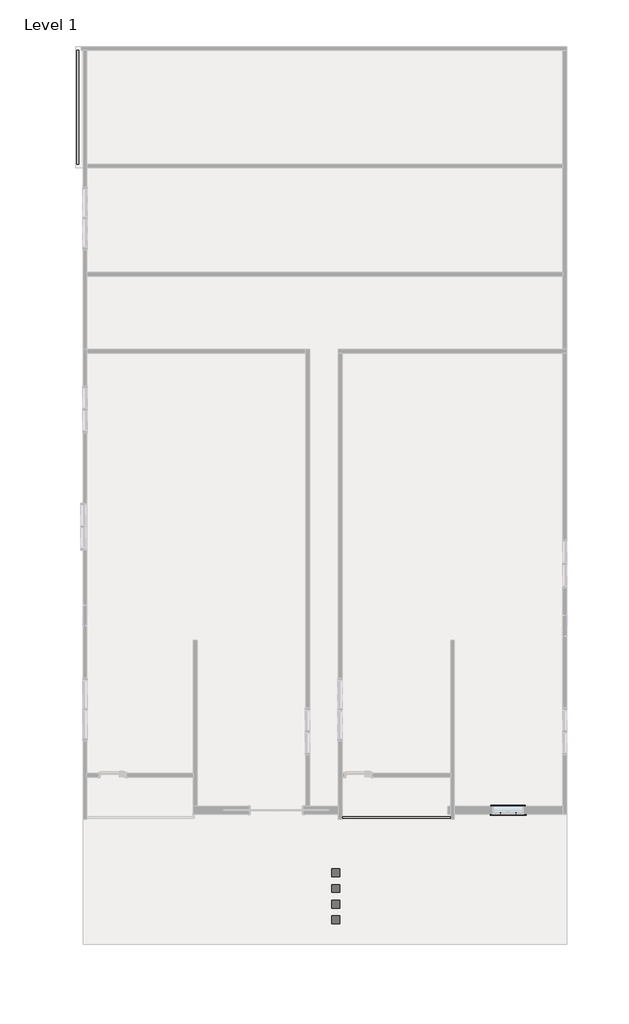
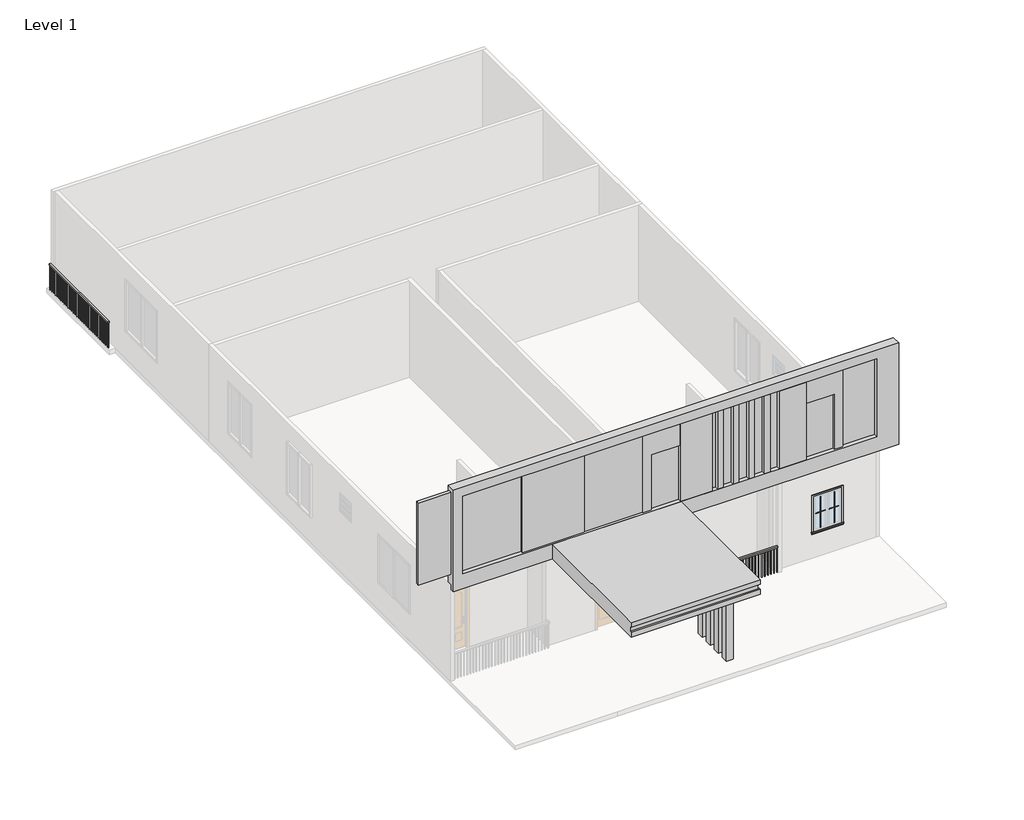
# One storey, part 3 of 3: 5 proxies, 3 railings.
"""IFC4 building model written with IfcOpenShell, lengths in millimetres."""

from ifc_helpers import new_model, si_unit, frame, origin, origin_with_axes, place, context, project, spatial, polyline, outline, extrude, transform, mapped, element, save
from components import generic_models_1_generic_models_1_486b888d, muntin_pattern_2x2_muntin_pattern_2x2_1acec82f, muntin_pattern_2x2_muntin_pattern_2x2_43d02eee, trim_window_exterior_flat_with_sill_e4b28ec3, trim_window_interior_flat_picture_frame_39ff4276

model = new_model("IFC4")

# Units and contexts
model_context = context("Model", 3, world=origin())
ifc_project = project(units=[si_unit("LENGTHUNIT", "METRE", prefix="MILLI")], contexts=[model_context])

# Site, building, storey
site = spatial("IfcSite", under=ifc_project)
building = spatial("IfcBuilding", under=site)
storey = spatial("IfcBuildingStorey", under=building, Name="Level 1", Elevation=0.0)

# Proxies
placement = place(None, origin())
generic_models_1_generic_models_1_shape = generic_models_1_generic_models_1_486b888d(model_context)
element("IfcBuildingElementProxy", 1, Name="Generic Models 1 : Generic Models 1", ObjectType="Generic Models 1 : Generic Models 1", at=placement, inside=storey, context=model_context, shape_type="MappedRepresentation", body=[
    mapped(generic_models_1_generic_models_1_shape, transform((0.0, 0.0, 0.0), x_axis=(1.0, 0.0, 0.0), y_axis=(0.0, 1.0, 0.0), z_axis=(0.0, 0.0, 1.0))),
])
muntin_pattern_2x2_muntin_pattern_2x2_shape = muntin_pattern_2x2_muntin_pattern_2x2_1acec82f(model_context)
element("IfcBuildingElementProxy", 2, Name="Muntin Pattern_2x2 : Muntin Pattern_2x2", ObjectType="Muntin Pattern_2x2 : Muntin Pattern_2x2", at=placement, inside=storey, context=model_context, shape_type="MappedRepresentation", body=[
    mapped(muntin_pattern_2x2_muntin_pattern_2x2_shape, transform((4424.1833786, -10576.3529557, 984.25), x_axis=(-1.0, 0.0, 0.0), y_axis=(0.0, -1.0, 0.0), z_axis=(0.0, 0.0, 1.0))),
])
muntin_pattern_2x2_muntin_pattern_2x2_2_shape = muntin_pattern_2x2_muntin_pattern_2x2_43d02eee(model_context)
element("IfcBuildingElementProxy", 3, Name="Muntin Pattern_2x2 : Muntin Pattern_2x2", ObjectType="Muntin Pattern_2x2 : Muntin Pattern_2x2", at=placement, inside=storey, context=model_context, shape_type="MappedRepresentation", body=[
    mapped(muntin_pattern_2x2_muntin_pattern_2x2_2_shape, transform((3970.1583786, -10576.3529557, 984.25), x_axis=(1.0, 0.0, 0.0), y_axis=(0.0, 1.0, 0.0), z_axis=(0.0, 0.0, 1.0))),
])
trim_window_exterior_flat_with_sill_shape = trim_window_exterior_flat_with_sill_e4b28ec3(model_context)
element("IfcBuildingElementProxy", 4, Name="Trim-Window-Exterior-Flat : with Sill", ObjectType="Trim-Window-Exterior-Flat : with Sill", at=placement, inside=storey, context=model_context, shape_type="MappedRepresentation", body=[
    mapped(trim_window_exterior_flat_with_sill_shape, transform((4197.1708786, -10585.8779557, 2133.6), x_axis=(1.0, 0.0, 0.0), y_axis=(0.0, 0.0, 1.0), z_axis=(0.0, -1.0, 0.0))),
])
trim_window_interior_flat_picture_frame_shape = trim_window_interior_flat_picture_frame_39ff4276(model_context)
element("IfcBuildingElementProxy", 5, Name="Trim-Window-Interior-Flat : Picture Frame", ObjectType="Trim-Window-Interior-Flat : Picture Frame", at=placement, inside=storey, context=model_context, shape_type="MappedRepresentation", body=[
    mapped(trim_window_interior_flat_picture_frame_shape, transform((4197.1708786, -10357.2779557, 2133.6), x_axis=(-1.0, 0.0, 0.0), y_axis=(0.0, 0.0, 1.0), z_axis=(0.0, 1.0, 0.0))),
])

# Railings
element("IfcRailing", 6, ObjectType="Handrail - Rectangular", at=placement, inside=storey, context=model_context, shape_type="SweptSolid", body=[
    extrude(outline(polyline([(-648.5431282, -10709.8005933), (-648.5431282, -10659.0005933), (2515.990751, -10659.0005933), (2515.990751, -10709.8005933), (-648.5431282, -10709.8005933)])), frame((0.0, 0.0, 863.6), z_axis=(0.0, 0.0, 1.0), x_axis=(1.0, 0.0, 0.0)), (0.0, 0.0, 1.0), 50.8),
    extrude(outline(polyline([(2491.5318718, -10693.9255933), (2491.5318718, -10674.8755933), (2510.5818718, -10674.8755933), (2510.5818718, -10693.9255933), (2491.5318718, -10693.9255933)])), origin_with_axes(), (0.0, 0.0, 1.0), 863.6),
    extrude(outline(polyline([(2389.9318718, -10693.9255933), (2389.9318718, -10674.8755933), (2408.9818718, -10674.8755933), (2408.9818718, -10693.9255933), (2389.9318718, -10693.9255933)])), origin_with_axes(), (0.0, 0.0, 1.0), 863.6),
    extrude(outline(polyline([(2288.3318718, -10693.9255933), (2288.3318718, -10674.8755933), (2307.3818718, -10674.8755933), (2307.3818718, -10693.9255933), (2288.3318718, -10693.9255933)])), origin_with_axes(), (0.0, 0.0, 1.0), 863.6),
    extrude(outline(polyline([(2186.7318718, -10693.9255933), (2186.7318718, -10674.8755933), (2205.7818718, -10674.8755933), (2205.7818718, -10693.9255933), (2186.7318718, -10693.9255933)])), origin_with_axes(), (0.0, 0.0, 1.0), 863.6),
    extrude(outline(polyline([(2085.1318718, -10693.9255933), (2085.1318718, -10674.8755933), (2104.1818718, -10674.8755933), (2104.1818718, -10693.9255933), (2085.1318718, -10693.9255933)])), origin_with_axes(), (0.0, 0.0, 1.0), 863.6),
    extrude(outline(polyline([(1983.5318718, -10693.9255933), (1983.5318718, -10674.8755933), (2002.5818718, -10674.8755933), (2002.5818718, -10693.9255933), (1983.5318718, -10693.9255933)])), origin_with_axes(), (0.0, 0.0, 1.0), 863.6),
    extrude(outline(polyline([(1881.9318718, -10693.9255933), (1881.9318718, -10674.8755933), (1900.9818718, -10674.8755933), (1900.9818718, -10693.9255933), (1881.9318718, -10693.9255933)])), origin_with_axes(), (0.0, 0.0, 1.0), 863.6),
    extrude(outline(polyline([(1780.3318718, -10693.9255933), (1780.3318718, -10674.8755933), (1799.3818718, -10674.8755933), (1799.3818718, -10693.9255933), (1780.3318718, -10693.9255933)])), origin_with_axes(), (0.0, 0.0, 1.0), 863.6),
    extrude(outline(polyline([(1678.7318718, -10693.9255933), (1678.7318718, -10674.8755933), (1697.7818718, -10674.8755933), (1697.7818718, -10693.9255933), (1678.7318718, -10693.9255933)])), origin_with_axes(), (0.0, 0.0, 1.0), 863.6),
    extrude(outline(polyline([(1577.1318718, -10693.9255933), (1577.1318718, -10674.8755933), (1596.1818718, -10674.8755933), (1596.1818718, -10693.9255933), (1577.1318718, -10693.9255933)])), origin_with_axes(), (0.0, 0.0, 1.0), 863.6),
    extrude(outline(polyline([(1475.5318718, -10693.9255933), (1475.5318718, -10674.8755933), (1494.5818718, -10674.8755933), (1494.5818718, -10693.9255933), (1475.5318718, -10693.9255933)])), origin_with_axes(), (0.0, 0.0, 1.0), 863.6),
    extrude(outline(polyline([(1373.9318718, -10693.9255933), (1373.9318718, -10674.8755933), (1392.9818718, -10674.8755933), (1392.9818718, -10693.9255933), (1373.9318718, -10693.9255933)])), origin_with_axes(), (0.0, 0.0, 1.0), 863.6),
    extrude(outline(polyline([(1272.3318718, -10693.9255933), (1272.3318718, -10674.8755933), (1291.3818718, -10674.8755933), (1291.3818718, -10693.9255933), (1272.3318718, -10693.9255933)])), origin_with_axes(), (0.0, 0.0, 1.0), 863.6),
    extrude(outline(polyline([(1170.7318718, -10693.9255933), (1170.7318718, -10674.8755933), (1189.7818718, -10674.8755933), (1189.7818718, -10693.9255933), (1170.7318718, -10693.9255933)])), origin_with_axes(), (0.0, 0.0, 1.0), 863.6),
    extrude(outline(polyline([(1069.1318718, -10693.9255933), (1069.1318718, -10674.8755933), (1088.1818718, -10674.8755933), (1088.1818718, -10693.9255933), (1069.1318718, -10693.9255933)])), origin_with_axes(), (0.0, 0.0, 1.0), 863.6),
    extrude(outline(polyline([(967.5318718, -10693.9255933), (967.5318718, -10674.8755933), (986.5818718, -10674.8755933), (986.5818718, -10693.9255933), (967.5318718, -10693.9255933)])), origin_with_axes(), (0.0, 0.0, 1.0), 863.6),
    extrude(outline(polyline([(865.9318718, -10693.9255933), (865.9318718, -10674.8755933), (884.9818718, -10674.8755933), (884.9818718, -10693.9255933), (865.9318718, -10693.9255933)])), origin_with_axes(), (0.0, 0.0, 1.0), 863.6),
    extrude(outline(polyline([(764.3318718, -10693.9255933), (764.3318718, -10674.8755933), (783.3818718, -10674.8755933), (783.3818718, -10693.9255933), (764.3318718, -10693.9255933)])), origin_with_axes(), (0.0, 0.0, 1.0), 863.6),
    extrude(outline(polyline([(662.7318718, -10693.9255933), (662.7318718, -10674.8755933), (681.7818718, -10674.8755933), (681.7818718, -10693.9255933), (662.7318718, -10693.9255933)])), origin_with_axes(), (0.0, 0.0, 1.0), 863.6),
    extrude(outline(polyline([(561.1318718, -10693.9255933), (561.1318718, -10674.8755933), (580.1818718, -10674.8755933), (580.1818718, -10693.9255933), (561.1318718, -10693.9255933)])), origin_with_axes(), (0.0, 0.0, 1.0), 863.6),
    extrude(outline(polyline([(459.5318718, -10693.9255933), (459.5318718, -10674.8755933), (478.5818718, -10674.8755933), (478.5818718, -10693.9255933), (459.5318718, -10693.9255933)])), origin_with_axes(), (0.0, 0.0, 1.0), 863.6),
    extrude(outline(polyline([(357.9318718, -10693.9255933), (357.9318718, -10674.8755933), (376.9818718, -10674.8755933), (376.9818718, -10693.9255933), (357.9318718, -10693.9255933)])), origin_with_axes(), (0.0, 0.0, 1.0), 863.6),
    extrude(outline(polyline([(256.3318718, -10693.9255933), (256.3318718, -10674.8755933), (275.3818718, -10674.8755933), (275.3818718, -10693.9255933), (256.3318718, -10693.9255933)])), origin_with_axes(), (0.0, 0.0, 1.0), 863.6),
    extrude(outline(polyline([(154.7318718, -10693.9255933), (154.7318718, -10674.8755933), (173.7818718, -10674.8755933), (173.7818718, -10693.9255933), (154.7318718, -10693.9255933)])), origin_with_axes(), (0.0, 0.0, 1.0), 863.6),
    extrude(outline(polyline([(53.1318718, -10693.9255933), (53.1318718, -10674.8755933), (72.1818718, -10674.8755933), (72.1818718, -10693.9255933), (53.1318718, -10693.9255933)])), origin_with_axes(), (0.0, 0.0, 1.0), 863.6),
    extrude(outline(polyline([(-48.4681282, -10693.9255933), (-48.4681282, -10674.8755933), (-29.4181282, -10674.8755933), (-29.4181282, -10693.9255933), (-48.4681282, -10693.9255933)])), origin_with_axes(), (0.0, 0.0, 1.0), 863.6),
    extrude(outline(polyline([(-150.0681282, -10693.9255933), (-150.0681282, -10674.8755933), (-131.0181282, -10674.8755933), (-131.0181282, -10693.9255933), (-150.0681282, -10693.9255933)])), origin_with_axes(), (0.0, 0.0, 1.0), 863.6),
    extrude(outline(polyline([(-251.6681282, -10693.9255933), (-251.6681282, -10674.8755933), (-232.6181282, -10674.8755933), (-232.6181282, -10693.9255933), (-251.6681282, -10693.9255933)])), origin_with_axes(), (0.0, 0.0, 1.0), 863.6),
    extrude(outline(polyline([(-353.2681282, -10693.9255933), (-353.2681282, -10674.8755933), (-334.2181282, -10674.8755933), (-334.2181282, -10693.9255933), (-353.2681282, -10693.9255933)])), origin_with_axes(), (0.0, 0.0, 1.0), 863.6),
    extrude(outline(polyline([(-454.8681282, -10693.9255933), (-454.8681282, -10674.8755933), (-435.8181282, -10674.8755933), (-435.8181282, -10693.9255933), (-454.8681282, -10693.9255933)])), origin_with_axes(), (0.0, 0.0, 1.0), 863.6),
    extrude(outline(polyline([(-556.4681282, -10693.9255933), (-556.4681282, -10674.8755933), (-537.4181282, -10674.8755933), (-537.4181282, -10693.9255933), (-556.4681282, -10693.9255933)])), origin_with_axes(), (0.0, 0.0, 1.0), 863.6),
    extrude(outline(polyline([(2496.940751, -10693.9255933), (2496.940751, -10674.8755933), (2515.990751, -10674.8755933), (2515.990751, -10693.9255933), (2496.940751, -10693.9255933)])), origin_with_axes(), (0.0, 0.0, 1.0), 863.6),
    extrude(outline(polyline([(-648.5431282, -10693.9255933), (-648.5431282, -10674.8755933), (-629.4931282, -10674.8755933), (-629.4931282, -10693.9255933), (-648.5431282, -10693.9255933)])), origin_with_axes(), (0.0, 0.0, 1.0), 863.6),
])
element("IfcRailing", 7, ObjectType="Handrail - Rectangular", at=placement, inside=storey, context=model_context, shape_type="SweptSolid", body=[
    extrude(outline(polyline([(-8391.7551246, 11703.9189683), (-8340.9551246, 11703.9189683), (-8340.9551246, 8387.4224771), (-8391.7551246, 8387.4224771), (-8391.7551246, 11703.9189683)])), frame((0.0, 0.0, 863.6), z_axis=(0.0, 0.0, 1.0), x_axis=(1.0, 0.0, 0.0)), (0.0, 0.0, 1.0), 50.8),
    extrude(outline(polyline([(-8375.8801246, 8462.2439683), (-8356.8301246, 8462.2439683), (-8356.8301246, 8443.1939683), (-8375.8801246, 8443.1939683), (-8375.8801246, 8462.2439683)])), origin_with_axes(), (0.0, 0.0, 1.0), 863.6),
    extrude(outline(polyline([(-8375.8801246, 8563.8439683), (-8356.8301246, 8563.8439683), (-8356.8301246, 8544.7939683), (-8375.8801246, 8544.7939683), (-8375.8801246, 8563.8439683)])), origin_with_axes(), (0.0, 0.0, 1.0), 863.6),
    extrude(outline(polyline([(-8375.8801246, 8665.4439683), (-8356.8301246, 8665.4439683), (-8356.8301246, 8646.3939683), (-8375.8801246, 8646.3939683), (-8375.8801246, 8665.4439683)])), origin_with_axes(), (0.0, 0.0, 1.0), 863.6),
    extrude(outline(polyline([(-8375.8801246, 8767.0439683), (-8356.8301246, 8767.0439683), (-8356.8301246, 8747.9939683), (-8375.8801246, 8747.9939683), (-8375.8801246, 8767.0439683)])), origin_with_axes(), (0.0, 0.0, 1.0), 863.6),
    extrude(outline(polyline([(-8375.8801246, 8868.6439683), (-8356.8301246, 8868.6439683), (-8356.8301246, 8849.5939683), (-8375.8801246, 8849.5939683), (-8375.8801246, 8868.6439683)])), origin_with_axes(), (0.0, 0.0, 1.0), 863.6),
    extrude(outline(polyline([(-8375.8801246, 8970.2439683), (-8356.8301246, 8970.2439683), (-8356.8301246, 8951.1939683), (-8375.8801246, 8951.1939683), (-8375.8801246, 8970.2439683)])), origin_with_axes(), (0.0, 0.0, 1.0), 863.6),
    extrude(outline(polyline([(-8375.8801246, 9071.8439683), (-8356.8301246, 9071.8439683), (-8356.8301246, 9052.7939683), (-8375.8801246, 9052.7939683), (-8375.8801246, 9071.8439683)])), origin_with_axes(), (0.0, 0.0, 1.0), 863.6),
    extrude(outline(polyline([(-8375.8801246, 9173.4439683), (-8356.8301246, 9173.4439683), (-8356.8301246, 9154.3939683), (-8375.8801246, 9154.3939683), (-8375.8801246, 9173.4439683)])), origin_with_axes(), (0.0, 0.0, 1.0), 863.6),
    extrude(outline(polyline([(-8375.8801246, 9275.0439683), (-8356.8301246, 9275.0439683), (-8356.8301246, 9255.9939683), (-8375.8801246, 9255.9939683), (-8375.8801246, 9275.0439683)])), origin_with_axes(), (0.0, 0.0, 1.0), 863.6),
    extrude(outline(polyline([(-8375.8801246, 9376.6439683), (-8356.8301246, 9376.6439683), (-8356.8301246, 9357.5939683), (-8375.8801246, 9357.5939683), (-8375.8801246, 9376.6439683)])), origin_with_axes(), (0.0, 0.0, 1.0), 863.6),
    extrude(outline(polyline([(-8375.8801246, 9478.2439683), (-8356.8301246, 9478.2439683), (-8356.8301246, 9459.1939683), (-8375.8801246, 9459.1939683), (-8375.8801246, 9478.2439683)])), origin_with_axes(), (0.0, 0.0, 1.0), 863.6),
    extrude(outline(polyline([(-8375.8801246, 9579.8439683), (-8356.8301246, 9579.8439683), (-8356.8301246, 9560.7939683), (-8375.8801246, 9560.7939683), (-8375.8801246, 9579.8439683)])), origin_with_axes(), (0.0, 0.0, 1.0), 863.6),
    extrude(outline(polyline([(-8375.8801246, 9681.4439683), (-8356.8301246, 9681.4439683), (-8356.8301246, 9662.3939683), (-8375.8801246, 9662.3939683), (-8375.8801246, 9681.4439683)])), origin_with_axes(), (0.0, 0.0, 1.0), 863.6),
    extrude(outline(polyline([(-8375.8801246, 9783.0439683), (-8356.8301246, 9783.0439683), (-8356.8301246, 9763.9939683), (-8375.8801246, 9763.9939683), (-8375.8801246, 9783.0439683)])), origin_with_axes(), (0.0, 0.0, 1.0), 863.6),
    extrude(outline(polyline([(-8375.8801246, 9884.6439683), (-8356.8301246, 9884.6439683), (-8356.8301246, 9865.5939683), (-8375.8801246, 9865.5939683), (-8375.8801246, 9884.6439683)])), origin_with_axes(), (0.0, 0.0, 1.0), 863.6),
    extrude(outline(polyline([(-8375.8801246, 9986.2439683), (-8356.8301246, 9986.2439683), (-8356.8301246, 9967.1939683), (-8375.8801246, 9967.1939683), (-8375.8801246, 9986.2439683)])), origin_with_axes(), (0.0, 0.0, 1.0), 863.6),
    extrude(outline(polyline([(-8375.8801246, 10087.8439683), (-8356.8301246, 10087.8439683), (-8356.8301246, 10068.7939683), (-8375.8801246, 10068.7939683), (-8375.8801246, 10087.8439683)])), origin_with_axes(), (0.0, 0.0, 1.0), 863.6),
    extrude(outline(polyline([(-8375.8801246, 10189.4439683), (-8356.8301246, 10189.4439683), (-8356.8301246, 10170.3939683), (-8375.8801246, 10170.3939683), (-8375.8801246, 10189.4439683)])), origin_with_axes(), (0.0, 0.0, 1.0), 863.6),
    extrude(outline(polyline([(-8375.8801246, 10291.0439683), (-8356.8301246, 10291.0439683), (-8356.8301246, 10271.9939683), (-8375.8801246, 10271.9939683), (-8375.8801246, 10291.0439683)])), origin_with_axes(), (0.0, 0.0, 1.0), 863.6),
    extrude(outline(polyline([(-8375.8801246, 10392.6439683), (-8356.8301246, 10392.6439683), (-8356.8301246, 10373.5939683), (-8375.8801246, 10373.5939683), (-8375.8801246, 10392.6439683)])), origin_with_axes(), (0.0, 0.0, 1.0), 863.6),
    extrude(outline(polyline([(-8375.8801246, 10494.2439683), (-8356.8301246, 10494.2439683), (-8356.8301246, 10475.1939683), (-8375.8801246, 10475.1939683), (-8375.8801246, 10494.2439683)])), origin_with_axes(), (0.0, 0.0, 1.0), 863.6),
    extrude(outline(polyline([(-8375.8801246, 10595.8439683), (-8356.8301246, 10595.8439683), (-8356.8301246, 10576.7939683), (-8375.8801246, 10576.7939683), (-8375.8801246, 10595.8439683)])), origin_with_axes(), (0.0, 0.0, 1.0), 863.6),
    extrude(outline(polyline([(-8375.8801246, 10697.4439683), (-8356.8301246, 10697.4439683), (-8356.8301246, 10678.3939683), (-8375.8801246, 10678.3939683), (-8375.8801246, 10697.4439683)])), origin_with_axes(), (0.0, 0.0, 1.0), 863.6),
    extrude(outline(polyline([(-8375.8801246, 10799.0439683), (-8356.8301246, 10799.0439683), (-8356.8301246, 10779.9939683), (-8375.8801246, 10779.9939683), (-8375.8801246, 10799.0439683)])), origin_with_axes(), (0.0, 0.0, 1.0), 863.6),
    extrude(outline(polyline([(-8375.8801246, 10900.6439683), (-8356.8301246, 10900.6439683), (-8356.8301246, 10881.5939683), (-8375.8801246, 10881.5939683), (-8375.8801246, 10900.6439683)])), origin_with_axes(), (0.0, 0.0, 1.0), 863.6),
    extrude(outline(polyline([(-8375.8801246, 11002.2439683), (-8356.8301246, 11002.2439683), (-8356.8301246, 10983.1939683), (-8375.8801246, 10983.1939683), (-8375.8801246, 11002.2439683)])), origin_with_axes(), (0.0, 0.0, 1.0), 863.6),
    extrude(outline(polyline([(-8375.8801246, 11103.8439683), (-8356.8301246, 11103.8439683), (-8356.8301246, 11084.7939683), (-8375.8801246, 11084.7939683), (-8375.8801246, 11103.8439683)])), origin_with_axes(), (0.0, 0.0, 1.0), 863.6),
    extrude(outline(polyline([(-8375.8801246, 11205.4439683), (-8356.8301246, 11205.4439683), (-8356.8301246, 11186.3939683), (-8375.8801246, 11186.3939683), (-8375.8801246, 11205.4439683)])), origin_with_axes(), (0.0, 0.0, 1.0), 863.6),
    extrude(outline(polyline([(-8375.8801246, 11307.0439683), (-8356.8301246, 11307.0439683), (-8356.8301246, 11287.9939683), (-8375.8801246, 11287.9939683), (-8375.8801246, 11307.0439683)])), origin_with_axes(), (0.0, 0.0, 1.0), 863.6),
    extrude(outline(polyline([(-8375.8801246, 11408.6439683), (-8356.8301246, 11408.6439683), (-8356.8301246, 11389.5939683), (-8375.8801246, 11389.5939683), (-8375.8801246, 11408.6439683)])), origin_with_axes(), (0.0, 0.0, 1.0), 863.6),
    extrude(outline(polyline([(-8375.8801246, 11510.2439683), (-8356.8301246, 11510.2439683), (-8356.8301246, 11491.1939683), (-8375.8801246, 11491.1939683), (-8375.8801246, 11510.2439683)])), origin_with_axes(), (0.0, 0.0, 1.0), 863.6),
    extrude(outline(polyline([(-8375.8801246, 11611.8439683), (-8356.8301246, 11611.8439683), (-8356.8301246, 11592.7939683), (-8375.8801246, 11592.7939683), (-8375.8801246, 11611.8439683)])), origin_with_axes(), (0.0, 0.0, 1.0), 863.6),
    extrude(outline(polyline([(-8375.8801246, 8406.4724771), (-8356.8301246, 8406.4724771), (-8356.8301246, 8387.4224771), (-8375.8801246, 8387.4224771), (-8375.8801246, 8406.4724771)])), origin_with_axes(), (0.0, 0.0, 1.0), 863.6),
    extrude(outline(polyline([(-8375.8801246, 11703.9189683), (-8356.8301246, 11703.9189683), (-8356.8301246, 11684.8689683), (-8375.8801246, 11684.8689683), (-8375.8801246, 11703.9189683)])), origin_with_axes(), (0.0, 0.0, 1.0), 863.6),
])
element("IfcRailing", 8, ObjectType="Handrail - Rectangular", at=placement, inside=storey, context=model_context, shape_type="SweptSolid", body=[
    extrude(outline(polyline([(5830.4721078, 11594.1725279), (5881.2721078, 11594.1725279), (5881.2721078, 8505.5262287), (5830.4721078, 8505.5262287), (5830.4721078, 11594.1725279)])), frame((0.0, 0.0, 863.6), z_axis=(0.0, 0.0, 1.0), x_axis=(1.0, 0.0, 0.0)), (0.0, 0.0, 1.0), 50.8),
    extrude(outline(polyline([(5846.3471078, 8555.6975279), (5865.3971078, 8555.6975279), (5865.3971078, 8536.6475279), (5846.3471078, 8536.6475279), (5846.3471078, 8555.6975279)])), origin_with_axes(), (0.0, 0.0, 1.0), 863.6),
    extrude(outline(polyline([(5846.3471078, 8657.2975279), (5865.3971078, 8657.2975279), (5865.3971078, 8638.2475279), (5846.3471078, 8638.2475279), (5846.3471078, 8657.2975279)])), origin_with_axes(), (0.0, 0.0, 1.0), 863.6),
    extrude(outline(polyline([(5846.3471078, 8758.8975279), (5865.3971078, 8758.8975279), (5865.3971078, 8739.8475279), (5846.3471078, 8739.8475279), (5846.3471078, 8758.8975279)])), origin_with_axes(), (0.0, 0.0, 1.0), 863.6),
    extrude(outline(polyline([(5846.3471078, 8860.4975279), (5865.3971078, 8860.4975279), (5865.3971078, 8841.4475279), (5846.3471078, 8841.4475279), (5846.3471078, 8860.4975279)])), origin_with_axes(), (0.0, 0.0, 1.0), 863.6),
    extrude(outline(polyline([(5846.3471078, 8962.0975279), (5865.3971078, 8962.0975279), (5865.3971078, 8943.0475279), (5846.3471078, 8943.0475279), (5846.3471078, 8962.0975279)])), origin_with_axes(), (0.0, 0.0, 1.0), 863.6),
    extrude(outline(polyline([(5846.3471078, 9063.6975279), (5865.3971078, 9063.6975279), (5865.3971078, 9044.6475279), (5846.3471078, 9044.6475279), (5846.3471078, 9063.6975279)])), origin_with_axes(), (0.0, 0.0, 1.0), 863.6),
    extrude(outline(polyline([(5846.3471078, 9165.2975279), (5865.3971078, 9165.2975279), (5865.3971078, 9146.2475279), (5846.3471078, 9146.2475279), (5846.3471078, 9165.2975279)])), origin_with_axes(), (0.0, 0.0, 1.0), 863.6),
    extrude(outline(polyline([(5846.3471078, 9266.8975279), (5865.3971078, 9266.8975279), (5865.3971078, 9247.8475279), (5846.3471078, 9247.8475279), (5846.3471078, 9266.8975279)])), origin_with_axes(), (0.0, 0.0, 1.0), 863.6),
    extrude(outline(polyline([(5846.3471078, 9368.4975279), (5865.3971078, 9368.4975279), (5865.3971078, 9349.4475279), (5846.3471078, 9349.4475279), (5846.3471078, 9368.4975279)])), origin_with_axes(), (0.0, 0.0, 1.0), 863.6),
    extrude(outline(polyline([(5846.3471078, 9470.0975279), (5865.3971078, 9470.0975279), (5865.3971078, 9451.0475279), (5846.3471078, 9451.0475279), (5846.3471078, 9470.0975279)])), origin_with_axes(), (0.0, 0.0, 1.0), 863.6),
    extrude(outline(polyline([(5846.3471078, 9571.6975279), (5865.3971078, 9571.6975279), (5865.3971078, 9552.6475279), (5846.3471078, 9552.6475279), (5846.3471078, 9571.6975279)])), origin_with_axes(), (0.0, 0.0, 1.0), 863.6),
    extrude(outline(polyline([(5846.3471078, 9673.2975279), (5865.3971078, 9673.2975279), (5865.3971078, 9654.2475279), (5846.3471078, 9654.2475279), (5846.3471078, 9673.2975279)])), origin_with_axes(), (0.0, 0.0, 1.0), 863.6),
    extrude(outline(polyline([(5846.3471078, 9774.8975279), (5865.3971078, 9774.8975279), (5865.3971078, 9755.8475279), (5846.3471078, 9755.8475279), (5846.3471078, 9774.8975279)])), origin_with_axes(), (0.0, 0.0, 1.0), 863.6),
    extrude(outline(polyline([(5846.3471078, 9876.4975279), (5865.3971078, 9876.4975279), (5865.3971078, 9857.4475279), (5846.3471078, 9857.4475279), (5846.3471078, 9876.4975279)])), origin_with_axes(), (0.0, 0.0, 1.0), 863.6),
    extrude(outline(polyline([(5846.3471078, 9978.0975279), (5865.3971078, 9978.0975279), (5865.3971078, 9959.0475279), (5846.3471078, 9959.0475279), (5846.3471078, 9978.0975279)])), origin_with_axes(), (0.0, 0.0, 1.0), 863.6),
    extrude(outline(polyline([(5846.3471078, 10079.6975279), (5865.3971078, 10079.6975279), (5865.3971078, 10060.6475279), (5846.3471078, 10060.6475279), (5846.3471078, 10079.6975279)])), origin_with_axes(), (0.0, 0.0, 1.0), 863.6),
    extrude(outline(polyline([(5846.3471078, 10181.2975279), (5865.3971078, 10181.2975279), (5865.3971078, 10162.2475279), (5846.3471078, 10162.2475279), (5846.3471078, 10181.2975279)])), origin_with_axes(), (0.0, 0.0, 1.0), 863.6),
    extrude(outline(polyline([(5846.3471078, 10282.8975279), (5865.3971078, 10282.8975279), (5865.3971078, 10263.8475279), (5846.3471078, 10263.8475279), (5846.3471078, 10282.8975279)])), origin_with_axes(), (0.0, 0.0, 1.0), 863.6),
    extrude(outline(polyline([(5846.3471078, 10384.4975279), (5865.3971078, 10384.4975279), (5865.3971078, 10365.4475279), (5846.3471078, 10365.4475279), (5846.3471078, 10384.4975279)])), origin_with_axes(), (0.0, 0.0, 1.0), 863.6),
    extrude(outline(polyline([(5846.3471078, 10486.0975279), (5865.3971078, 10486.0975279), (5865.3971078, 10467.0475279), (5846.3471078, 10467.0475279), (5846.3471078, 10486.0975279)])), origin_with_axes(), (0.0, 0.0, 1.0), 863.6),
    extrude(outline(polyline([(5846.3471078, 10587.6975279), (5865.3971078, 10587.6975279), (5865.3971078, 10568.6475279), (5846.3471078, 10568.6475279), (5846.3471078, 10587.6975279)])), origin_with_axes(), (0.0, 0.0, 1.0), 863.6),
    extrude(outline(polyline([(5846.3471078, 10689.2975279), (5865.3971078, 10689.2975279), (5865.3971078, 10670.2475279), (5846.3471078, 10670.2475279), (5846.3471078, 10689.2975279)])), origin_with_axes(), (0.0, 0.0, 1.0), 863.6),
    extrude(outline(polyline([(5846.3471078, 10790.8975279), (5865.3971078, 10790.8975279), (5865.3971078, 10771.8475279), (5846.3471078, 10771.8475279), (5846.3471078, 10790.8975279)])), origin_with_axes(), (0.0, 0.0, 1.0), 863.6),
    extrude(outline(polyline([(5846.3471078, 10892.4975279), (5865.3971078, 10892.4975279), (5865.3971078, 10873.4475279), (5846.3471078, 10873.4475279), (5846.3471078, 10892.4975279)])), origin_with_axes(), (0.0, 0.0, 1.0), 863.6),
    extrude(outline(polyline([(5846.3471078, 10994.0975279), (5865.3971078, 10994.0975279), (5865.3971078, 10975.0475279), (5846.3471078, 10975.0475279), (5846.3471078, 10994.0975279)])), origin_with_axes(), (0.0, 0.0, 1.0), 863.6),
    extrude(outline(polyline([(5846.3471078, 11095.6975279), (5865.3971078, 11095.6975279), (5865.3971078, 11076.6475279), (5846.3471078, 11076.6475279), (5846.3471078, 11095.6975279)])), origin_with_axes(), (0.0, 0.0, 1.0), 863.6),
    extrude(outline(polyline([(5846.3471078, 11197.2975279), (5865.3971078, 11197.2975279), (5865.3971078, 11178.2475279), (5846.3471078, 11178.2475279), (5846.3471078, 11197.2975279)])), origin_with_axes(), (0.0, 0.0, 1.0), 863.6),
    extrude(outline(polyline([(5846.3471078, 11298.8975279), (5865.3971078, 11298.8975279), (5865.3971078, 11279.8475279), (5846.3471078, 11279.8475279), (5846.3471078, 11298.8975279)])), origin_with_axes(), (0.0, 0.0, 1.0), 863.6),
    extrude(outline(polyline([(5846.3471078, 11400.4975279), (5865.3971078, 11400.4975279), (5865.3971078, 11381.4475279), (5846.3471078, 11381.4475279), (5846.3471078, 11400.4975279)])), origin_with_axes(), (0.0, 0.0, 1.0), 863.6),
    extrude(outline(polyline([(5846.3471078, 11502.0975279), (5865.3971078, 11502.0975279), (5865.3971078, 11483.0475279), (5846.3471078, 11483.0475279), (5846.3471078, 11502.0975279)])), origin_with_axes(), (0.0, 0.0, 1.0), 863.6),
    extrude(outline(polyline([(5846.3471078, 8524.5762287), (5865.3971078, 8524.5762287), (5865.3971078, 8505.5262287), (5846.3471078, 8505.5262287), (5846.3471078, 8524.5762287)])), origin_with_axes(), (0.0, 0.0, 1.0), 863.6),
    extrude(outline(polyline([(5846.3471078, 11594.1725279), (5865.3971078, 11594.1725279), (5865.3971078, 11575.1225279), (5846.3471078, 11575.1225279), (5846.3471078, 11594.1725279)])), origin_with_axes(), (0.0, 0.0, 1.0), 863.6),
])

save(model, "model.ifc")

# Revit data of these elements
# Type "Muntin Pattern_2x2 : Muntin Pattern_2x2"
#   Width [instance default] = 4' - 0"
#   Thickness = 0' - 0 1/2"
#   Height [instance default] = 4' - 0"
#   Distance = 0' - 0 3/4"
#   Interior Material [instance default] = none
#   Exterior Material [instance default] = none
#   Default Elevation = 0
# Type "Trim-Window-Exterior-Flat : with Sill"
#   Trim Width = 0' - 2 1/4"
#   Trim Thickness_Picture Frame = 0' - 1 1/4"
#   Trim Thickness_with Sill = 0' - 0 3/4"
#   Sill Thickness = 0' - 1 1/4"
#   Opening Width [instance default] = 2' - 0"
#   Opening Height [instance default] = 3' - 0"
#   Default Elevation = 4' - 0"
#   Sill = yes
#   Picture Frame = no
#   Trim Material [instance default] = none
# Type "Trim-Window-Interior-Flat : Picture Frame"
#   Trim Thickness_Picture Frame = 0' - 1 1/4"
#   Trim Width = 0' - 2 1/4"
#   Trim Thickness_with Sill = 0' - 0 3/4"
#   Sill Thickness = 0' - 1 1/4"
#   Opening Width [instance default] = 2' - 0"
#   Opening Height [instance default] = 3' - 0"
#   Default Elevation = 4' - 0"
#   Sill = no
#   Picture Frame = yes
#   Trim Material [instance default] = none
# Type "Handrail - Rectangular"
#   Assembly Code = "C2010400"
#   built-in parameter 1008612 = 0.0416667 (stored number, unit not read)
#   built-in parameter 1008611 = 0.0416667 (stored number, unit not read)
#   built-in parameter 1008609 = 0.333333 (stored number, unit not read)
#   built-in parameter 1008604 = 0.166667 (stored number, unit not read)
#   built-in parameter 1008603 = 0.166667 (stored number, unit not read)
#   Railing Height = 3' - 0"
#   built-in parameter 1008630 = 2
#   built-in parameter 1008610 = 2
#   built-in parameter 1008618 = Baluster - Square : 3/4"
# Element 1 (IfcBuildingElementProxy, "Generic Models 1 : Generic Models 1")
#   Phase Created = New Construction
#   Materials on its faces: "Gypsum Wall Board", "wood", "Water"
# Elements 2, 3 (IfcBuildingElementProxy, "Muntin Pattern_2x2 : Muntin Pattern_2x2")
#   Width = 1' - 0 5/8"
#   Height = 3' - 6 1/2"
#   Interior Material = Wood - Stained
#   Exterior Material = Clad - White
#   Phase Created = New Construction
#   Materials on its faces: "Clad - White", "Wood - Stained"
# Element 4 (IfcBuildingElementProxy, "Trim-Window-Exterior-Flat : with Sill")
#   Opening Width = 3' - 0"
#   Opening Height = 4' - 0"
#   Trim Material = Clad - White
#   Phase Created = New Construction
#   Materials on its faces: "Clad - White"
# Element 5 (IfcBuildingElementProxy, "Trim-Window-Interior-Flat : Picture Frame")
#   Opening Width = 3' - 0"
#   Opening Height = 4' - 0"
#   Trim Material = Wood - Stained
#   Phase Created = New Construction
#   Materials on its faces: "Wood - Stained"
# Elements 6, 7, 8 (IfcRailing, "Handrail - Rectangular")
#   Phase Created = New Construction
# Materials
#   "Gypsum Wall Board": class "Generic", colour RGB 127 127 127, transparency 0, Description = "Gypsum Wall Board", Cost = 0
#   "wood": class "Generic", colour RGB 120 120 120, transparency 0, Cost = 0
#   "Water": class "Liquid", colour RGB 108 195 217, transparency 0.7, Description = "Water", Cost = 0
#   "Clad - White": class "Wood", colour RGB 242 242 238, transparency 0, Cost = 0
#   "Wood - Stained": class "Wood", colour RGB 224 178 126, transparency 0, Cost = 0
